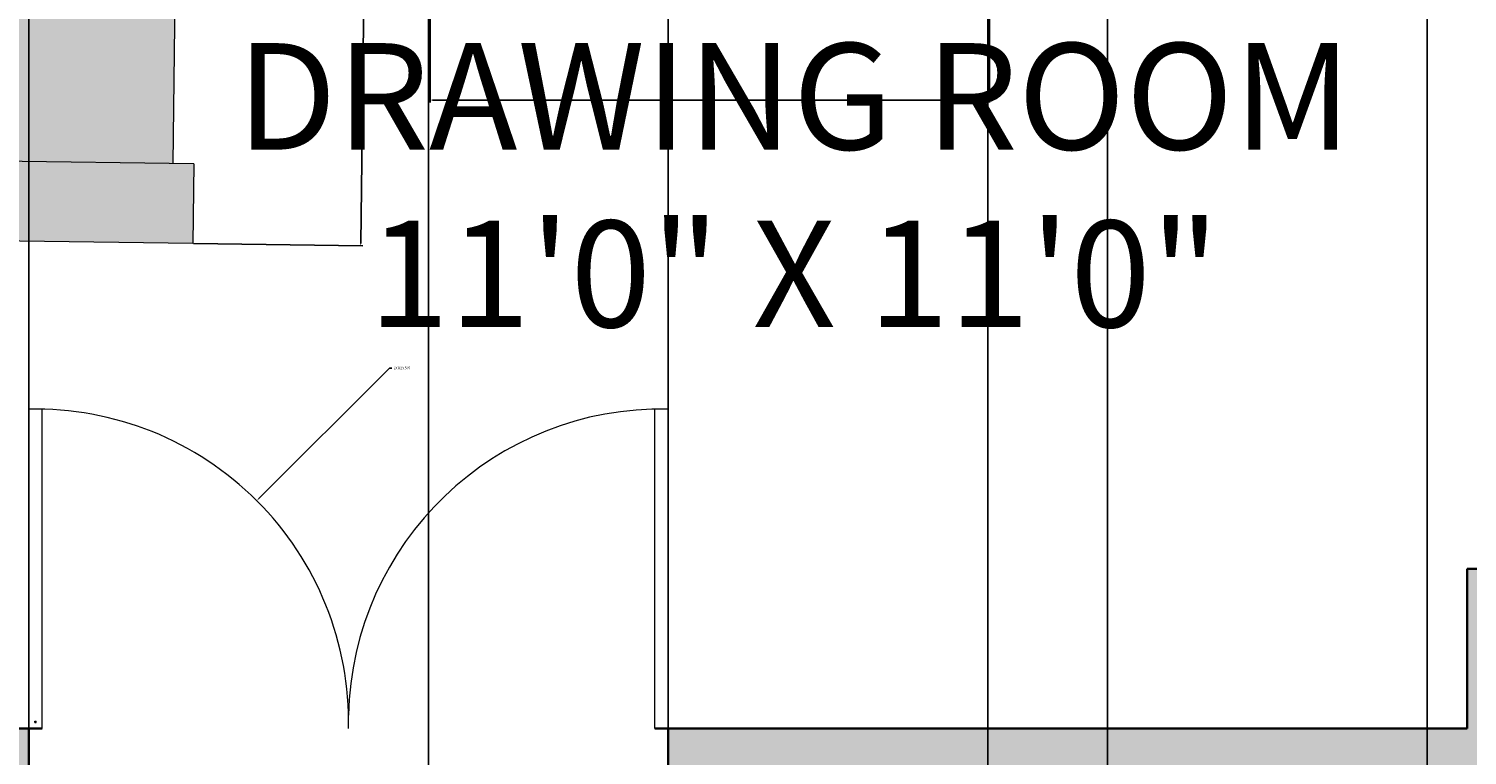
# Model space of a CAD drawing. Units: inches. Extents: x 1567 to 1964, y 1813 to 2447.
# Tile 8 of 28: x 1630 to 1738, y 2125 to 2180. Entities that reach past the tile are written whole.
import ezdxf

# ---------------------------------------------------------------- set-up
doc = ezdxf.new("R2010")
doc.units = ezdxf.units.IN
for name, color, linetype, lineweight in [('A-ANNO-DIMS', 2, 'Continuous', 18), ('A-AREA-IDEN', 7, 'Continuous', 18), ('A-DOOR', 4, 'Continuous', 18), ('A-FURN', 8, 'Continuous', 18), ('A-WALL', 7, 'Continuous', 35)]:
    doc.layers.add(name, color=color, linetype=linetype, lineweight=lineweight)
doc.layers.add('A-FURN-PATT', color=252, linetype='Continuous', lineweight=13, true_color=0x939598)
doc.layers.add('A-WALL-PATT', color=251, linetype='Continuous', lineweight=13, true_color=0x636466)
doc.styles.get("Standard").update_dxf_attribs({"font": 'arial.ttf'})
doc.dimstyles.get("Standard").update_dxf_attribs({"dimtxt": 0.18, "dimasz": 0.18, "dimexe": 0.18, "dimexo": 0.0625, "dimgap": 0.09, "dimtad": 0, "dimtih": 1, "dimtoh": 1, "dimdec": 4, "dimzin": 0, "dimdsep": 46, "dimtxsty": 'Standard', "dimcen": 0.09, "dimadec": 0, "dimazin": 0, "dimtfac": 1, "dimtdec": 4, "dimtofl": 0, "dimtmove": 0, "dimatfit": 3, "dimfxl": 1, "dimtolj": 1, "dimtzin": 0, "dimarcsym": 0})

# ---------------------------------------------------------------- blocks, each defined once
blk = doc.blocks.new('Sofa - Roundback 7 ft.')
for p, q in [((-12.00002, -32.4421), (-12.00003, -6.5971)), ((11.99997, -32.4421), (11.99998, -6.5971)), ((-36.000027, -34), (-36.000027, -11.4696)), ((35.99998, -34), (35.99998, -11.4696)), ((-35.999844, -13.3819), (35.9998, -13.3819)), ((-36.000027, -32.4421), (35.99998, -32.4421))]:
    blk.add_line(p, q)
for points in [[(-36.000027, -34), (-42.000027, -34), (-42.000027, -8)], [(41.99998, -8), (41.99998, -34), (35.99998, -34)]]:
    blk.add_lwpolyline(points)
for centre, radius, start, end in [((0, -114.25), 114.25, 68.43141, 111.5686), ((-0.00001, -127.1968), 121.1968, 72.72033, 107.2797)]:
    blk.add_arc(centre, radius, start, end)
blk = doc.blocks.new('*D23')
at = {"layer": 'A-ANNO-DIMS', "color": 0, "lineweight": -2, "transparency": 16777216}
for p, q in [((1643.92, 2247.72), (1656.64, 2247.55)), ((1656.46, 2247.38), (1655.9, 2205.74)), ((1655.35, 2163.74), (1655.9, 2205.38)), ((1642.81, 2163.73), (1655.52, 2163.56))]:
    blk.add_line(p, q, dxfattribs=at)
at = {"layer": 'A-ANNO-DIMS', "color": 0, "transparency": 16777216}
for points in [[(1656.43, 2247.38), (1656.49, 2247.38), (1656.46, 2247.56)], [(1655.32, 2163.74), (1655.38, 2163.74), (1655.34, 2163.56)]]:
    blk.add_solid(points, dxfattribs=at)
at = {"layer": 'Defpoints', "color": 0, "transparency": 16777216}
for p in [(1643.86, 2247.72), (1656.46, 2247.56), (1642.75, 2163.73)]:
    blk.add_point(p, dxfattribs=at)
at = {"layer": 'A-ANNO-DIMS', "color": 0, "transparency": 16777216, "insert": (1655.9, 2205.56), "char_height": 0.18, "attachment_point": 5}
blk.add_mtext('\\A1;SOFA 84', dxfattribs=at)
blk = doc.blocks.new('*D26')
at = {"layer": 'A-ANNO-DIMS', "color": 0, "lineweight": -2, "transparency": 16777216}
for p, q in [((1660.56, 2180.74), (1660.56, 2174.33)), ((1702.56, 2180.74), (1702.56, 2174.33)), ((1660.74, 2174.51), (1681.34, 2174.51)), ((1702.38, 2174.51), (1681.78, 2174.51))]:
    blk.add_line(p, q, dxfattribs=at)
at = {"layer": 'A-ANNO-DIMS', "color": 0, "transparency": 16777216}
for points in [[(1660.74, 2174.54), (1660.74, 2174.48), (1660.56, 2174.51)], [(1702.38, 2174.54), (1702.38, 2174.48), (1702.56, 2174.51)]]:
    blk.add_solid(points, dxfattribs=at)
at = {"layer": 'Defpoints', "color": 0, "transparency": 16777216}
for p in [(1660.56, 2180.81), (1702.56, 2180.81), (1702.56, 2174.51)]:
    blk.add_point(p, dxfattribs=at)
at = {"layer": 'A-ANNO-DIMS', "color": 0, "transparency": 16777216, "insert": (1681.56, 2174.51), "char_height": 0.18, "attachment_point": 5}
blk.add_mtext('\\A1;42', dxfattribs=at)
blk = doc.blocks.new('*D54')
at = {"layer": 'A-ANNO-DIMS', "color": 0, "lineweight": -2, "transparency": 16777216}
for p, q in [((1711.43, 1964.35), (1711.43, 2447.12)), ((1711.61, 2446.94), (1753.21, 2446.94)), ((1795.25, 2446.94), (1753.65, 2446.94)), ((1795.43, 1964.35), (1795.43, 2447.12))]:
    blk.add_line(p, q, dxfattribs=at)
at = {"layer": 'A-ANNO-DIMS', "color": 0, "transparency": 16777216}
for points in [[(1711.61, 2446.97), (1711.61, 2446.91), (1711.43, 2446.94)], [(1795.25, 2446.97), (1795.25, 2446.91), (1795.43, 2446.94)]]:
    blk.add_solid(points, dxfattribs=at)
at = {"layer": 'Defpoints', "color": 0, "transparency": 16777216}
for p in [(1795.43, 2446.94), (1711.43, 1964.29), (1795.43, 1964.29)]:
    blk.add_point(p, dxfattribs=at)
at = {"layer": 'A-ANNO-DIMS', "color": 0, "transparency": 16777216, "insert": (1753.43, 2446.94), "char_height": 0.18, "attachment_point": 5}
blk.add_mtext('\\A1;84', dxfattribs=at)
blk = doc.blocks.new('*D57')
at = {"layer": 'A-ANNO-DIMS', "color": 0, "lineweight": -2, "transparency": 16777216}
for p, q in [((1630.43, 2127.35), (1630.43, 2447.12)), ((1630.61, 2446.94), (1654.21, 2446.94)), ((1678.25, 2446.94), (1654.65, 2446.94)), ((1678.43, 2127.35), (1678.43, 2447.12))]:
    blk.add_line(p, q, dxfattribs=at)
at = {"layer": 'A-ANNO-DIMS', "color": 0, "transparency": 16777216}
for points in [[(1630.61, 2446.97), (1630.61, 2446.91), (1630.43, 2446.94)], [(1678.25, 2446.97), (1678.25, 2446.91), (1678.43, 2446.94)]]:
    blk.add_solid(points, dxfattribs=at)
at = {"layer": 'Defpoints', "color": 0, "transparency": 16777216}
for p in [(1678.43, 2446.94), (1630.43, 2127.29), (1678.43, 2127.29)]:
    blk.add_point(p, dxfattribs=at)
at = {"layer": 'A-ANNO-DIMS', "color": 0, "transparency": 16777216, "insert": (1654.43, 2446.94), "char_height": 0.18, "attachment_point": 5}
blk.add_mtext('\\A1;48', dxfattribs=at)
blk = doc.blocks.new('*D60')
at = {"layer": 'A-ANNO-DIMS', "color": 0, "lineweight": -2, "transparency": 16777216}
for p, q in [((1660.43, 2063.35), (1660.43, 2447.12)), ((1660.61, 2446.94), (1681.21, 2446.94)), ((1702.25, 2446.94), (1681.65, 2446.94)), ((1702.43, 2063.35), (1702.43, 2447.12))]:
    blk.add_line(p, q, dxfattribs=at)
at = {"layer": 'A-ANNO-DIMS', "color": 0, "transparency": 16777216}
for points in [[(1660.61, 2446.97), (1660.61, 2446.91), (1660.43, 2446.94)], [(1702.25, 2446.97), (1702.25, 2446.91), (1702.43, 2446.94)]]:
    blk.add_solid(points, dxfattribs=at)
at = {"layer": 'Defpoints', "color": 0, "transparency": 16777216}
for p in [(1660.43, 2446.94), (1660.43, 2063.29), (1702.43, 2063.29)]:
    blk.add_point(p, dxfattribs=at)
at = {"layer": 'A-ANNO-DIMS', "color": 0, "transparency": 16777216, "insert": (1681.43, 2446.94), "char_height": 0.18, "attachment_point": 5}
blk.add_mtext('\\A1;42', dxfattribs=at)
blk = doc.blocks.new('*D63')
at = {"layer": 'A-ANNO-DIMS', "color": 0, "lineweight": -2, "transparency": 16777216}
for p, q in [((1735.43, 1988.35), (1735.43, 2447.12)), ((1735.61, 2446.94), (1753.21, 2446.94)), ((1771.25, 2446.94), (1753.65, 2446.94)), ((1771.43, 1988.35), (1771.43, 2447.12))]:
    blk.add_line(p, q, dxfattribs=at)
at = {"layer": 'A-ANNO-DIMS', "color": 0, "transparency": 16777216}
for points in [[(1735.61, 2446.97), (1735.61, 2446.91), (1735.43, 2446.94)], [(1771.25, 2446.97), (1771.25, 2446.91), (1771.43, 2446.94)]]:
    blk.add_solid(points, dxfattribs=at)
at = {"layer": 'Defpoints', "color": 0, "transparency": 16777216}
for p in [(1771.43, 2446.94), (1735.43, 1988.29), (1771.43, 1988.29)]:
    blk.add_point(p, dxfattribs=at)
at = {"layer": 'A-ANNO-DIMS', "color": 0, "transparency": 16777216, "insert": (1753.43, 2446.94), "char_height": 0.18, "attachment_point": 5}
blk.add_mtext('\\A1;36', dxfattribs=at)
blk = doc.blocks.new('*D64')
at = {"layer": 'A-ANNO-DIMS', "color": 0, "lineweight": -2, "transparency": 16777216}
for p, q in [((1711.43, 2055.85), (1711.43, 2447.12)), ((1711.61, 2446.94), (1723.21, 2446.94)), ((1735.25, 2446.94), (1723.65, 2446.94)), ((1735.43, 2055.85), (1735.43, 2447.12))]:
    blk.add_line(p, q, dxfattribs=at)
at = {"layer": 'A-ANNO-DIMS', "color": 0, "transparency": 16777216}
for points in [[(1711.61, 2446.97), (1711.61, 2446.91), (1711.43, 2446.94)], [(1735.25, 2446.97), (1735.25, 2446.91), (1735.43, 2446.94)]]:
    blk.add_solid(points, dxfattribs=at)
at = {"layer": 'Defpoints', "color": 0, "transparency": 16777216}
for p in [(1735.43, 2446.94), (1711.43, 2055.79), (1735.43, 2055.79)]:
    blk.add_point(p, dxfattribs=at)
at = {"layer": 'A-ANNO-DIMS', "color": 0, "transparency": 16777216, "insert": (1723.43, 2446.94), "char_height": 0.18, "attachment_point": 5}
blk.add_mtext('\\A1;24', dxfattribs=at)
blk = doc.blocks.new('*D73')
at = {"layer": 'A-ANNO-DIMS', "color": 0, "lineweight": -2, "transparency": 16777216}
for p, q in [((1657.52, 2154.38), (1647.68, 2144.54)), ((1657.7, 2154.38), (1657.52, 2154.38)), ((1630.84, 2127.79), (1631.02, 2127.79)), ((1630.93, 2127.7), (1630.93, 2127.88))]:
    blk.add_line(p, q, dxfattribs=at)
at = {"layer": 'A-ANNO-DIMS', "color": 0, "transparency": 16777216}
blk.add_solid([(1647.66, 2144.56), (1647.7, 2144.52), (1647.55, 2144.41)], dxfattribs=at)
at = {"layer": 'Defpoints', "color": 0, "transparency": 16777216}
for p in [(1647.55, 2144.41), (1630.93, 2127.79)]:
    blk.add_point(p, dxfattribs=at)
at = {"layer": 'A-ANNO-DIMS', "color": 0, "transparency": 16777216, "insert": (1658.45, 2154.38), "char_height": 0.18, "attachment_point": 5}
blk.add_mtext('\\A1;2X R23.505', dxfattribs=at)

msp = doc.modelspace()

# ---------------------------------------------------------------- hatches: boundary and pattern name
at = {"layer": 'A-FURN-PATT'}
h = msp.add_hatch(color=256, dxfattribs=at)
h.dxf.hatch_style = 1
h.paths.add_polyline_path([(1621.2532, 2242.0229), (1643.7811, 2241.7239), (1643.8607, 2247.7234), (1617.863, 2248.0685, 0.19047621), (1616.7481, 2164.0759), (1642.7458, 2163.7308), (1642.8254, 2169.7302), (1620.2975, 2170.0293, -0.15194781)])
h.paths.add_polyline_path([(1673.5306, 2249.6607), (1653.8509, 2249.6607), (1653.8509, 2248.5031, 0.11764706), (1673.5306, 2248.5031)])
h.paths.add_polyline_path([(1706.0889, 2249.6607), (1686.4092, 2249.6607), (1686.4092, 2248.5031, 0.11764706), (1706.0889, 2248.5031)])
h.paths.add_polyline_path([(1782.4511, 2227.4197), (1766.4511, 2227.4197), (1766.2949, 2226.4197), (1782.6074, 2226.4197)])
h.paths.add_polyline_path([(1810.4511, 2227.4197), (1794.4511, 2227.4197), (1794.2949, 2226.4197), (1810.6074, 2226.4197)])
h.paths.add_polyline_path([(1743.9511, 2208.076), (1742.9511, 2207.9197), (1742.9511, 2191.9197), (1743.9511, 2191.7635)])
h.paths.add_polyline_path([(1782.6074, 2173.4197), (1766.2949, 2173.4197), (1766.4511, 2172.4197), (1782.4511, 2172.4197)])
h.paths.add_polyline_path([(1810.6074, 2173.4197), (1794.2949, 2173.4197), (1794.4511, 2172.4197), (1810.4511, 2172.4197)])
h.paths.add_polyline_path([(1861.053, 2006.5071), (1845.8531, 2006.5071), (1861.053, 1991.3071)])
h.paths.add_polyline_path([(1905.853, 1993.7071), (1861.053, 1993.7071), (1861.053, 1991.3071), (1905.853, 1991.3071)])
h.paths.add_polyline_path([(1919.7245, 2257.29, 0.50000012), (1918.7245, 2258.29), (1901.7245, 2258.29, 0.50000012), (1900.7245, 2257.29), (1900.7245, 2253.29, 0.50000012), (1901.7245, 2252.29), (1918.7245, 2252.29, 0.50000012), (1919.7245, 2253.29)])
h.paths.add_polyline_path([(1875.9094, 2391.0204), (1875.9094, 2375.8204), (1891.1093, 2375.8204)], flags=17)
h.paths.add_polyline_path([(1891.1093, 2405.4204), (1831.1094, 2405.4204), (1831.1094, 2391.0204), (1839.1093, 2391.0204), (1839.1093, 2404.2204), (1859.9093, 2404.2204), (1859.9093, 2391.0204), (1862.3093, 2391.0204), (1862.3093, 2404.2204), (1883.1093, 2404.2204), (1883.1093, 2389.0204), (1877.9094, 2389.0204), (1891.1093, 2375.8204)])
h.paths.add_polyline_path([(1682.1402, 2390.0316), (1682.1402, 2374.8316), (1697.3402, 2374.8316)], flags=17)
h.paths.add_polyline_path([(1697.3402, 2404.4316), (1637.3402, 2404.4316), (1637.3402, 2390.0316), (1645.3402, 2390.0316), (1645.3402, 2403.2316), (1666.1402, 2403.2316), (1666.1402, 2390.0316), (1668.5402, 2390.0316), (1668.5402, 2403.2316), (1689.3402, 2403.2316), (1689.3402, 2388.0316), (1684.1402, 2388.0316), (1697.3402, 2374.8316)])
h = msp.add_hatch(color=256, dxfattribs=at)
h.dxf.hatch_style = 1
h.paths.add_polyline_path([(1642.2233, 2241.7446), (1623.1648, 2241.9976), (1622.8462, 2217.9997), (1641.9047, 2217.7467)])
h.paths.add_polyline_path([(1641.9047, 2217.7467), (1622.8462, 2217.9997), (1622.5277, 2194.0018), (1641.5862, 2193.7488)])
h.paths.add_polyline_path([(1641.5862, 2193.7488), (1622.5277, 2194.0018), (1622.2091, 2170.0039), (1641.2677, 2169.7509)])
h.paths.add_polyline_path([(1671.2154, 2243.8726, -0.23606798), (1673.5306, 2245.0302), (1673.5306, 2246.1879), (1653.8509, 2246.1879), (1653.8509, 2245.0302, -0.23606798), (1656.1662, 2243.8726), (1656.1662, 2233.4539, -0.23606798), (1653.8509, 2232.2963), (1653.8509, 2231.1387, 0.11764706), (1673.5306, 2231.1387), (1673.5306, 2232.2963, -0.23606798), (1671.2154, 2233.4539)])
h.paths.add_polyline_path([(1703.7736, 2243.8726, -0.23606798), (1706.0889, 2245.0302), (1706.0889, 2246.1879), (1686.4092, 2246.1879), (1686.4092, 2245.0302, -0.23606798), (1688.7245, 2243.8726), (1688.7245, 2233.4539, -0.23606798), (1686.4092, 2232.2963), (1686.4092, 2231.1387, 0.11764706), (1706.0889, 2231.1387), (1706.0889, 2232.2963, -0.23606798), (1703.7736, 2233.4539)])
h.paths.add_polyline_path([(1782.6855, 2225.9197), (1766.2168, 2225.9197), (1764.9668, 2217.9197), (1783.9356, 2217.9197)])
h.paths.add_polyline_path([(1810.6855, 2225.9197), (1794.2168, 2225.9197), (1792.9668, 2217.9197), (1811.9356, 2217.9197)])
h.paths.add_polyline_path([(1752.4511, 2209.4041), (1744.4511, 2208.1541), (1744.4511, 2191.6853), (1752.4511, 2190.4354)])
h.paths.add_polyline_path([(1783.9356, 2181.9197), (1764.9668, 2181.9197), (1766.2168, 2173.9197), (1782.6855, 2173.9197)])
h.paths.add_polyline_path([(1811.9356, 2181.9197), (1792.9668, 2181.9197), (1794.2168, 2173.9197), (1810.6855, 2173.9197)])
h.paths.add_polyline_path([(1832.4511, 2208.1541), (1824.4511, 2209.4041), (1824.4511, 2190.4354), (1832.4511, 2191.6853)])
h.paths.add_polyline_path([(1824.4511, 2194.4197), (1823.8775, 2194.266), (1823.2838, 2194.1743), (1822.6735, 2194.1363), (1822.0501, 2194.1437), (1821.4169, 2194.1882), (1820.7773, 2194.2615), (1820.1348, 2194.3554), (1819.4928, 2194.4614), (1818.8527, 2194.5726), (1818.2083, 2194.6873), (1817.5511, 2194.8049), (1816.873, 2194.9249), (1816.1656, 2195.0469), (1815.4205, 2195.1704), (1814.6296, 2195.2948), (1813.7845, 2195.4197), (1812.88, 2195.5442), (1811.9238, 2195.6658), (1810.9265, 2195.7815), (1809.899, 2195.8885), (1808.852, 2195.9837), (1807.7962, 2196.0643), (1806.7423, 2196.1273), (1805.7011, 2196.1697), (1804.6806, 2196.1896), (1803.6777, 2196.188), (1802.6865, 2196.1668), (1801.7011, 2196.1281), (1800.7158, 2196.0737), (1799.7245, 2196.0057), (1798.7216, 2195.9259), (1797.7011, 2195.8364), (1796.6564, 2195.7387), (1795.5781, 2195.6333), (1794.4557, 2195.52), (1793.2792, 2195.3989), (1792.0383, 2195.27), (1790.7226, 2195.1333), (1789.3219, 2194.9887), (1787.8261, 2194.8364), (1786.1882, 2194.6764), (1784.2148, 2194.5096), (1781.6759, 2194.3369), (1778.3417, 2194.1593), (1773.9821, 2193.9778), (1768.3671, 2193.7934), (1761.2668, 2193.6071), (1752.4511, 2193.4197), (1752.4511, 2189.9197), (1762.0489, 2190.1067), (1769.9836, 2190.2908), (1776.4672, 2190.469), (1781.7115, 2190.6385), (1785.9285, 2190.7962), (1789.33, 2190.9393), (1792.128, 2191.0648), (1794.5344, 2191.1697), (1796.7278, 2191.2521), (1798.7532, 2191.313), (1800.6223, 2191.3543), (1802.3469, 2191.3781), (1803.9387, 2191.3862), (1805.4094, 2191.3807), (1806.7708, 2191.3634), (1808.0345, 2191.3364), (1809.2127, 2191.3013), (1810.3196, 2191.2589), (1811.3699, 2191.2097), (1812.3782, 2191.1541), (1813.3592, 2191.0927), (1814.3274, 2191.0259), (1815.2976, 2190.9542), (1816.2845, 2190.8781), (1817.2985, 2190.7986), (1818.3339, 2190.7186), (1819.3811, 2190.6415), (1820.4303, 2190.5708), (1821.4716, 2190.5098), (1822.4954, 2190.4621), (1823.4918, 2190.4309), (1824.3581, 2190.4208), (1824.4511, 2190.4354)])
h.paths.add_polyline_path([(1874.6531, 1991.3071), (1861.053, 1991.3071), (1859.053, 1993.3071), (1853.8531, 1993.3071), (1853.8531, 1978.1071), (1874.6531, 1978.1071)], flags=17)
h.paths.add_polyline_path([(1897.8531, 1991.3071), (1877.0531, 1991.3071), (1877.0531, 1978.1071), (1897.8531, 1978.1071)], flags=17)
h.paths.add_polyline_path([(1853.8531, 1993.3071), (1859.053, 1993.3071), (1845.8531, 2006.5071), (1845.8531, 1976.9071), (1905.853, 1976.9071), (1905.853, 1991.3071), (1897.8531, 1991.3071), (1897.8531, 1978.1071), (1877.0531, 1978.1071), (1877.0531, 1991.3071), (1874.6531, 1991.3071), (1874.6531, 1978.1071), (1853.8531, 1978.1071)])
h.paths.add_polyline_path([(1920.7245, 2259.29), (1899.7245, 2259.29), (1899.7245, 2251.29), (1920.7245, 2251.29)])
h.paths.add_polyline_path([(1918.7245, 2252.29, 0.50000012), (1919.7245, 2253.29), (1919.7245, 2257.29, 0.50000012), (1918.7245, 2258.29), (1901.7245, 2258.29, 0.50000012), (1900.7245, 2257.29), (1900.7245, 2253.29, 0.50000012), (1901.7245, 2252.29)], flags=16)
h.paths.add_polyline_path([(1843.2327, 2065.967), (1919.26, 2065.967), (1919.26, 2095.8187), (1843.2327, 2095.8187)], flags=9)
at = {"layer": 'A-WALL-PATT'}
h = msp.add_hatch(color=256, dxfattribs=at)
h.dxf.hatch_style = 1
h.paths.add_polyline_path([(1606.4295, 2407.29), (1654.4295, 2407.29), (1654.4295, 2416.29), (1597.4295, 2416.29), (1597.4295, 2217.29), (1606.4295, 2217.29), (1606.4295, 2259.29), (1738.4295, 2259.29), (1738.4295, 2247.29), (1742.4295, 2247.29), (1742.4295, 2259.29), (1742.4295, 2272.29), (1738.4295, 2272.29), (1738.4295, 2263.29), (1606.4295, 2263.29)])
h.paths.add_polyline_path([(1753.4295, 2416.29), (1690.4295, 2416.29), (1690.4295, 2407.29), (1738.4295, 2407.29), (1738.4295, 2308.29), (1742.4295, 2308.29), (1742.4295, 2331.29), (1746.9295, 2331.29), (1746.9295, 2335.29), (1742.4295, 2335.29), (1742.4295, 2407.29), (1753.4295, 2407.29)])
h.paths.add_polyline_path([(1840.4295, 2416.29), (1777.4295, 2416.29), (1777.4295, 2407.29), (1788.4295, 2407.29), (1788.4295, 2335.29), (1776.9295, 2335.29), (1776.9295, 2331.29), (1788.4295, 2331.29), (1788.4295, 2308.29), (1792.4295, 2308.29), (1792.4295, 2407.29), (1840.4295, 2407.29)])
h.paths.add_polyline_path([(1933.4295, 2416.29), (1876.4295, 2416.29), (1876.4295, 2407.29), (1924.4295, 2407.29), (1924.4295, 2263.29), (1792.4295, 2263.29), (1792.4295, 2272.29), (1788.4295, 2272.29), (1788.4295, 2259.29), (1872.4295, 2259.29), (1872.4295, 2171.29), (1880.9295, 2171.29), (1880.9295, 2175.29), (1876.4295, 2175.29), (1876.4295, 2259.29), (1924.4295, 2259.29), (1924.4295, 2229.29), (1933.4295, 2229.29)])
h.paths.add_polyline_path([(1933.4295, 2205.29), (1924.4295, 2205.29), (1924.4295, 2175.29), (1910.9295, 2175.29), (1910.9295, 2171.29), (1924.4295, 2171.29), (1924.4295, 2127.29), (1844.4295, 2127.29), (1844.4295, 2123.29), (1924.4295, 2123.29), (1924.4295, 2063.29), (1933.4295, 2063.29)])
h.paths.add_polyline_path([(1799.4295, 2123.29), (1808.4295, 2123.29), (1808.4295, 2127.29), (1781.4295, 2127.29), (1781.4295, 2123.29), (1795.4295, 2123.29), (1795.4295, 1964.29), (1711.4295, 1964.29), (1711.4295, 2123.29), (1751.4295, 2123.29), (1751.4295, 2127.29), (1742.4295, 2127.29), (1742.4295, 2139.29), (1738.4295, 2139.29), (1738.4295, 2127.29), (1678.4295, 2127.29), (1678.4295, 2123.29), (1702.4295, 2123.29), (1702.4295, 1913.29), (1678.4295, 1913.29), (1678.4295, 1904.29), (1711.4295, 1904.29), (1711.4295, 1960.29), (1795.4295, 1960.29), (1795.4295, 1906.69), (1929.4295, 1906.69), (1929.4295, 1848.29), (1601.4295, 1848.29), (1601.4295, 1904.29), (1630.4295, 1904.29), (1630.4295, 1913.29), (1606.4295, 1913.29), (1606.4295, 2123.29), (1630.4295, 2123.29), (1630.4295, 2127.29), (1606.4295, 2127.29), (1606.4295, 2169.29), (1597.4295, 2169.29), (1597.4295, 1844.29), (1933.4295, 1844.29), (1933.4295, 2027.29), (1924.4295, 2027.29), (1924.4295, 1967.29), (1833.9295, 1967.29), (1833.9295, 1963.29), (1924.4295, 1963.29), (1924.4295, 1910.69), (1799.4295, 1910.69), (1799.4295, 1963.29), (1803.9295, 1963.29), (1803.9295, 1967.29), (1799.4295, 1967.29)])

# ---------------------------------------------------------------- linework, layer by layer
at = {"layer": 'A-DOOR'}
for p, q in [((1630.4295, 2127.29), (1630.4295, 2151.29)), ((1631.4295, 2127.29), (1631.4295, 2151.29)), ((1677.4295, 2127.29), (1677.4295, 2151.29)), ((1678.4295, 2127.29), (1678.4295, 2151.29))]:
    msp.add_line(p, q, dxfattribs=at)
for centre, start, end in [((1630.9295, 2127.79), 358.781125, 91.218875), ((1677.9295, 2127.79), 88.781125, 178.781125)]:
    msp.add_arc(centre, 23.5053, start, end, dxfattribs=at)
at = {"layer": 'A-WALL'}
for p, q in [((1738.4295, 2127.29), (1738.4295, 2139.29)), ((1738.4295, 2139.29), (1742.4295, 2139.29)), ((1606.4295, 2127.29), (1631.4295, 2127.29)), ((1630.4295, 2123.29), (1630.4295, 2127.29)), ((1677.4295, 2127.29), (1738.4295, 2127.29)), ((1678.4295, 2123.29), (1678.4295, 2127.29))]:
    msp.add_line(p, q, dxfattribs=at)

# ---------------------------------------------------------------- block references
at = {"layer": 'A-FURN', "rotation": 89.2395118843373}
msp.add_blockref('Sofa - Roundback 7 ft.', (1609.3062, 2206.1784), dxfattribs=at)

# ---------------------------------------------------------------- texts
at = {"layer": 'A-AREA-IDEN', "insert": (1629.0764, 2178.7848), "char_height": 8, "attachment_point": 1}
msp.add_mtext_dynamic_manual_height_columns('\\pxqc;DRAWING ROOM\\P11\'0" X 11\'0"', width=117.636737, gutter_width=12.5, heights=[0], dxfattribs=at)

# ---------------------------------------------------------------- dimensions: what is measured, and where the dimension line sits
at = {"layer": 'A-ANNO-DIMS'}
for base, p1, p2, picture, middle in [((1678.4295, 2446.94), (1630.4295, 2127.29), (1678.4295, 2127.29), '*D57', (1654.4295, 2446.94)), ((1660.4295, 2446.94), (1702.4295, 2063.29), (1660.4295, 2063.29), '*D60', (1681.4295, 2446.94)), ((1795.4295, 2446.94), (1711.4295, 1964.29), (1795.4295, 1964.29), '*D54', (1753.4295, 2446.94)), ((1735.4295, 2446.94), (1711.4295, 2055.79), (1735.4295, 2055.79), '*D64', (1723.4295, 2446.94)), ((1771.4295, 2446.94), (1735.4295, 1988.29), (1771.4295, 1988.29), '*D63', (1753.4295, 2446.94)), ((1702.5611, 2174.5054), (1660.5611, 2180.8057), (1702.5611, 2180.8057), '*D26', (1681.5611, 2174.5054))]:
    dim = msp.add_linear_dim(base=base, p1=p1, p2=p2, dimstyle='Standard', override={"dimdec": 0, "dimlfac": 1, "dimrnd": 0, "dimzin": 0, "dimdsep": 46, "dimlunit": 2}, dxfattribs=at)
    dim.commit()
    dim.dimension.update_dxf_attribs({"geometry": picture, "text_midpoint": middle})
dim = msp.add_linear_dim(base=(1656.4596, 2247.5562), p1=(1642.7458, 2163.7308), p2=(1643.8607, 2247.7234), angle=89.239512, text='SOFA <>', dimstyle='Standard', override={"dimdec": 0, "dimlfac": 1, "dimrnd": 0, "dimzin": 0, "dimdsep": 46, "dimlunit": 2}, dxfattribs=at)
dim.commit()
dim.dimension.update_dxf_attribs({"geometry": '*D23', "text_midpoint": (1655.9021, 2205.5598)})
dim = msp.add_radius_dim(center=(1630.9295, 2127.79), mpoint=(1647.55, 2144.411), text='2X <>', dimstyle='Standard', override={"dimdec": 3, "dimlfac": 1, "dimrnd": 0, "dimzin": 0, "dimdsep": 46, "dimlunit": 2}, dxfattribs=at)
dim.commit()
dim.dimension.update_dxf_attribs({"geometry": '*D73', "text_midpoint": (1658.4477, 2154.3837), "dimtype": 164})

doc.saveas('drawing.dxf')
